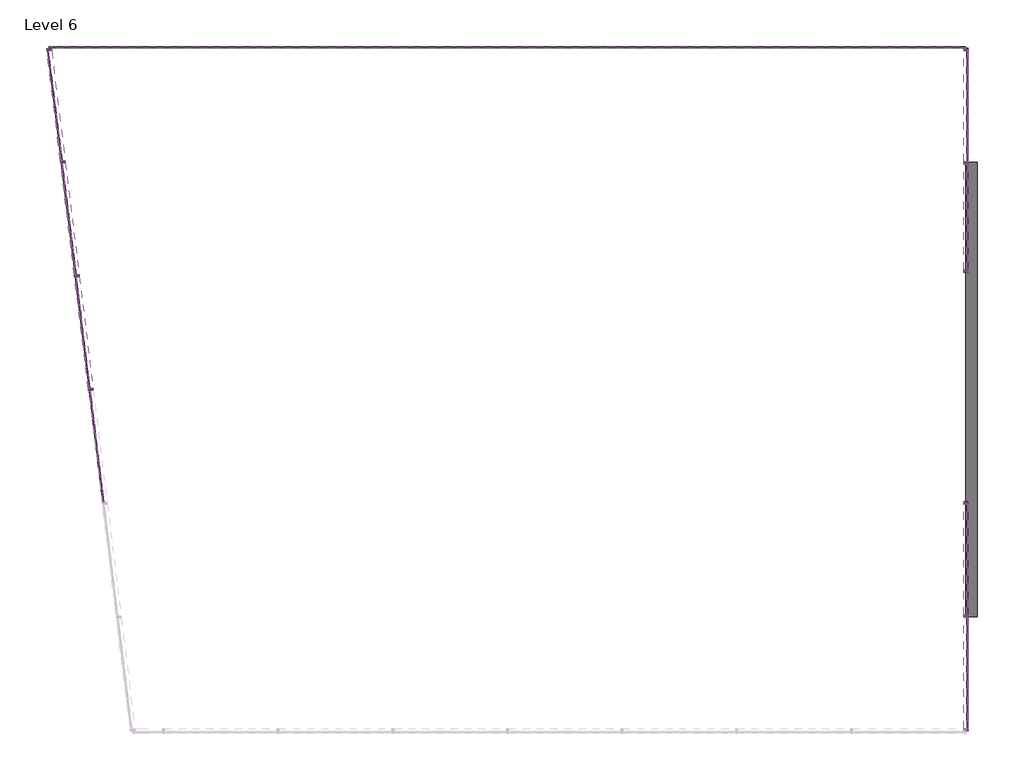
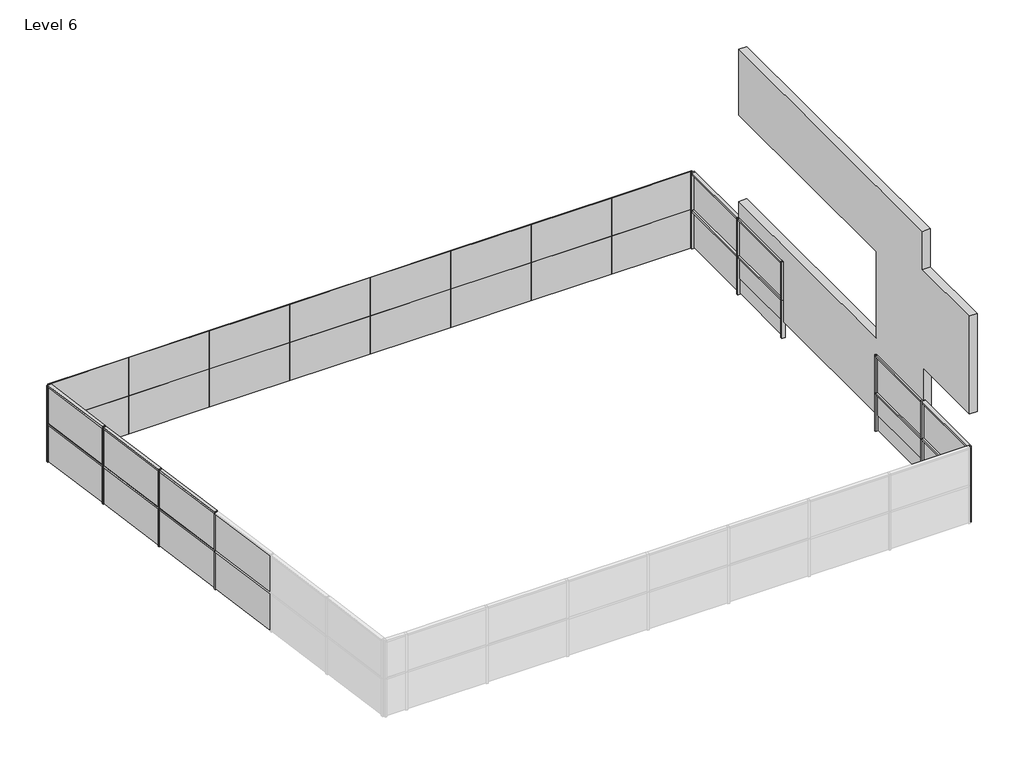
# One storey, part 2 of 2: 34 members, 32 plates, 1 proxy.
"""IFC4 building model written with IfcOpenShell, lengths in millimetres."""

from ifc_helpers import new_model, si_unit, origin, place, context, project, spatial, transform, mapped, element, save
from components import generic_models_3_generic_models_1_fe68d0d7, member_daa7a266, member_82905deb, member_19d0a4ec, member_8cef0660, member_4491d118, member_46bdb8c2, member_1b94d493, system_panel_glazed_1e57f9bb, system_panel_glazed_37f15d2e, system_panel_glazed_e46d4b42, system_panel_glazed_2a6c68b7, system_panel_glazed_7fb1fc2b, system_panel_glazed_d483336f

model = new_model("IFC4")

# Units and contexts
model_context = context("Model", 3, world=origin())
ifc_project = project(units=[si_unit("LENGTHUNIT", "METRE", prefix="MILLI")], contexts=[model_context])

# Site, building, storey
site = spatial("IfcSite", under=ifc_project)
building = spatial("IfcBuilding", under=site)
storey = spatial("IfcBuildingStorey", under=building, Name="Level 6", Elevation=15240.0)

# Proxy
placement = place(None, origin())
generic_models_3_generic_models_1_shape = generic_models_3_generic_models_1_fe68d0d7(model_context)
element("IfcBuildingElementProxy", 1, Name="Generic Models 3 : Generic Models 1", ObjectType="Generic Models 3 : Generic Models 1", at=placement, inside=storey, context=model_context, shape_type="MappedRepresentation", body=[
    mapped(generic_models_3_generic_models_1_shape, transform((0.0, 0.0, 17373.6), x_axis=(1.0, 0.0, 0.0), y_axis=(0.0, 1.0, 0.0), z_axis=(0.0, 0.0, 1.0))),
])

# Members
member_shape = member_daa7a266(model_context)
element("IfcMember", 2, ObjectType="Rectangular Mullion : 2.5\" x 5\" rectangular", at=placement, inside=storey, context=model_context, shape_type="MappedRepresentation", body=[
    mapped(member_shape, transform((13902.5156363, -946.6363705, 18288.0), x_axis=(0.0, 0.0, 1.0), y_axis=(1.0, 0.0, 0.0), z_axis=(0.0, 1.0, 0.0))),
])
element("IfcMember", 3, ObjectType="Rectangular Mullion : 2.5\" x 5\" rectangular", at=placement, inside=storey, context=model_context, shape_type="MappedRepresentation", body=[
    mapped(member_shape, transform((13902.5156363, -3962.8863708, 18288.0), x_axis=(0.0, 0.0, 1.0), y_axis=(1.0, 0.0, 0.0), z_axis=(0.0, 1.0, 0.0))),
])
element("IfcMember", 4, ObjectType="Rectangular Mullion : 2.5\" x 5\" rectangular", at=placement, inside=storey, context=model_context, shape_type="MappedRepresentation", body=[
    mapped(member_shape, transform((13902.5156363, 11109.0476508, 18288.0), x_axis=(0.0, 0.0, 1.0), y_axis=(1.0, 0.0, 0.0), z_axis=(0.0, 1.0, 0.0))),
])
member_2_shape = member_82905deb(model_context)
element("IfcMember", 5, ObjectType="Rectangular Mullion : 2.5\" x 5\" rectangular", at=placement, inside=storey, context=model_context, shape_type="MappedRepresentation", body=[
    mapped(member_2_shape, transform((13902.5156363, -3931.1363708, 18288.0), x_axis=(0.0, -1.0, 0.0), y_axis=(1.0, 0.0, 0.0), z_axis=(0.0, 0.0, 1.0))),
])
element("IfcMember", 6, ObjectType="Rectangular Mullion : 2.5\" x 5\" rectangular", at=placement, inside=storey, context=model_context, shape_type="MappedRepresentation", body=[
    mapped(member_2_shape, transform((13902.5156363, 8124.5476505, 18288.0), x_axis=(0.0, -1.0, 0.0), y_axis=(1.0, 0.0, 0.0), z_axis=(0.0, 0.0, 1.0))),
])
member_3_shape = member_19d0a4ec(model_context)
element("IfcMember", 7, ObjectType="Rectangular Mullion : 2.5\" x 5\" rectangular", at=placement, inside=storey, context=model_context, shape_type="MappedRepresentation", body=[
    mapped(member_3_shape, transform((-10113.8959567, 8178.7803212, 16764.0), x_axis=(0.0, 0.0, 1.0), y_axis=(-0.9925461516413222, -0.12186934340514609, 0.0), z_axis=(0.12186934340514609, -0.9925461516413222, 0.0))),
])
element("IfcMember", 8, ObjectType="Rectangular Mullion : 2.5\" x 5\" rectangular", at=placement, inside=storey, context=model_context, shape_type="MappedRepresentation", body=[
    mapped(member_3_shape, transform((-10113.8959567, 8178.7803212, 18288.0), x_axis=(0.0, 0.0, 1.0), y_axis=(-0.9925461516413222, -0.12186934340514617, 0.0), z_axis=(0.12186934340514617, -0.9925461516413222, 0.0))),
])
element("IfcMember", 9, ObjectType="Rectangular Mullion : 2.5\" x 5\" rectangular", at=placement, inside=storey, context=model_context, shape_type="MappedRepresentation", body=[
    mapped(member_3_shape, transform((13902.5156363, -946.6363705, 16764.0), x_axis=(0.0, 0.0, 1.0), y_axis=(1.0, 0.0, 0.0), z_axis=(0.0, 1.0, 0.0))),
])
element("IfcMember", 10, ObjectType="Rectangular Mullion : 2.5\" x 5\" rectangular", at=placement, inside=storey, context=model_context, shape_type="MappedRepresentation", body=[
    mapped(member_3_shape, transform((13902.5156363, -3962.8863708, 16764.0), x_axis=(0.0, 0.0, 1.0), y_axis=(1.0, 0.0, 0.0), z_axis=(0.0, 1.0, 0.0))),
])
element("IfcMember", 11, ObjectType="Rectangular Mullion : 2.5\" x 5\" rectangular", at=placement, inside=storey, context=model_context, shape_type="MappedRepresentation", body=[
    mapped(member_3_shape, transform((13902.5156363, 11109.0476508, 16764.0), x_axis=(0.0, 0.0, 1.0), y_axis=(1.0, 0.0, 0.0), z_axis=(0.0, 1.0, 0.0))),
])
member_4_shape = member_8cef0660(model_context)
element("IfcMember", 12, ObjectType="Rectangular Mullion : 2.5\" x 5\" rectangular", at=placement, inside=storey, context=model_context, shape_type="MappedRepresentation", body=[
    mapped(member_4_shape, transform((-9370.9804393, 2128.2189808, 16764.0), x_axis=(0.0, 0.0, 1.0), y_axis=(-0.9925461516413223, -0.12186934340514563, 0.0), z_axis=(0.12186934340514562, -0.9925461516413222, 0.0))),
])
element("IfcMember", 13, ObjectType="Rectangular Mullion : 2.5\" x 5\" rectangular", at=placement, inside=storey, context=model_context, shape_type="MappedRepresentation", body=[
    mapped(member_4_shape, transform((-9742.438198, 5153.499651, 16764.0), x_axis=(0.0, 0.0, 1.0), y_axis=(-0.9925461516413222, -0.12186934340514602, 0.0), z_axis=(0.12186934340514602, -0.9925461516413222, 0.0))),
])
element("IfcMember", 14, ObjectType="Rectangular Mullion : 2.5\" x 5\" rectangular", at=placement, inside=storey, context=model_context, shape_type="MappedRepresentation", body=[
    mapped(member_4_shape, transform((-9370.9804393, 2128.2189808, 18288.0), x_axis=(0.0, 0.0, 1.0), y_axis=(-0.9925461516413222, -0.12186934340514592, 0.0), z_axis=(0.12186934340514592, -0.9925461516413222, 0.0))),
])
element("IfcMember", 15, ObjectType="Rectangular Mullion : 2.5\" x 5\" rectangular", at=placement, inside=storey, context=model_context, shape_type="MappedRepresentation", body=[
    mapped(member_4_shape, transform((-9742.438198, 5153.499651, 18288.0), x_axis=(0.0, 0.0, 1.0), y_axis=(-0.9925461516413222, -0.1218693434051457, 0.0), z_axis=(0.1218693434051457, -0.9925461516413222, 0.0))),
])
element("IfcMember", 16, ObjectType="Rectangular Mullion : 2.5\" x 5\" rectangular", at=placement, inside=storey, context=model_context, shape_type="MappedRepresentation", body=[
    mapped(member_2_shape, transform((-9367.1110876, 2096.7056405, 16764.0), x_axis=(-0.1218693434051459, 0.9925461516413222, 0.0), y_axis=(-0.9925461516413222, -0.1218693434051459, 0.0), z_axis=(0.0, 0.0, 1.0))),
])
element("IfcMember", 17, ObjectType="Rectangular Mullion : 2.5\" x 5\" rectangular", at=placement, inside=storey, context=model_context, shape_type="MappedRepresentation", body=[
    mapped(member_2_shape, transform((-9367.1110876, 2096.7056405, 18288.0), x_axis=(-0.1218693434051459, 0.9925461516413222, 0.0), y_axis=(-0.9925461516413222, -0.1218693434051459, 0.0), z_axis=(0.0, 0.0, 1.0))),
])
element("IfcMember", 18, ObjectType="Rectangular Mullion : 2.5\" x 5\" rectangular", at=placement, inside=storey, context=model_context, shape_type="MappedRepresentation", body=[
    mapped(member_2_shape, transform((-9738.5688463, 5121.9863107, 16764.0), x_axis=(-0.1218693434051459, 0.9925461516413222, 0.0), y_axis=(-0.9925461516413222, -0.1218693434051459, 0.0), z_axis=(0.0, 0.0, 1.0))),
])
element("IfcMember", 19, ObjectType="Rectangular Mullion : 2.5\" x 5\" rectangular", at=placement, inside=storey, context=model_context, shape_type="MappedRepresentation", body=[
    mapped(member_2_shape, transform((-9738.5688463, 5121.9863107, 18288.0), x_axis=(-0.1218693434051459, 0.9925461516413222, 0.0), y_axis=(-0.9925461516413222, -0.1218693434051459, 0.0), z_axis=(0.0, 0.0, 1.0))),
])
element("IfcMember", 20, ObjectType="Rectangular Mullion : 2.5\" x 5\" rectangular", at=placement, inside=storey, context=model_context, shape_type="MappedRepresentation", body=[
    mapped(member_2_shape, transform((-10110.026605, 8147.2669809, 16764.0), x_axis=(-0.1218693434051459, 0.9925461516413222, 0.0), y_axis=(-0.9925461516413222, -0.1218693434051459, 0.0), z_axis=(0.0, 0.0, 1.0))),
])
element("IfcMember", 21, ObjectType="Rectangular Mullion : 2.5\" x 5\" rectangular", at=placement, inside=storey, context=model_context, shape_type="MappedRepresentation", body=[
    mapped(member_2_shape, transform((-10110.026605, 8147.2669809, 18288.0), x_axis=(-0.1218693434051459, 0.9925461516413222, 0.0), y_axis=(-0.9925461516413222, -0.1218693434051459, 0.0), z_axis=(0.0, 0.0, 1.0))),
])
element("IfcMember", 22, ObjectType="Rectangular Mullion : 2.5\" x 5\" rectangular", at=placement, inside=storey, context=model_context, shape_type="MappedRepresentation", body=[
    mapped(member_2_shape, transform((13902.5156363, -3931.1363708, 16764.0), x_axis=(0.0, -1.0, 0.0), y_axis=(1.0, 0.0, 0.0), z_axis=(0.0, 0.0, 1.0))),
])
element("IfcMember", 23, ObjectType="Rectangular Mullion : 2.5\" x 5\" rectangular", at=placement, inside=storey, context=model_context, shape_type="MappedRepresentation", body=[
    mapped(member_2_shape, transform((13902.5156363, 8124.5476505, 16764.0), x_axis=(0.0, -1.0, 0.0), y_axis=(1.0, 0.0, 0.0), z_axis=(0.0, 0.0, 1.0))),
])
member_5_shape = member_4491d118(model_context)
element("IfcMember", 24, ObjectType="Rectangular Mullion : 2.5\" x 5\" rectangular", at=placement, inside=storey, context=model_context, shape_type="MappedRepresentation", body=[
    mapped(member_5_shape, transform((13902.5156363, -6979.1363705, 18288.0), x_axis=(0.0, -1.0, 0.0), y_axis=(1.0, 0.0, 0.0), z_axis=(0.0, 0.0, 1.0))),
])
element("IfcMember", 25, ObjectType="Rectangular Mullion : 2.5\" x 5\" rectangular", at=placement, inside=storey, context=model_context, shape_type="MappedRepresentation", body=[
    mapped(member_5_shape, transform((13902.5156363, 5212.8636295, 18288.0), x_axis=(0.0, -1.0, 0.0), y_axis=(1.0, 0.0, 0.0), z_axis=(0.0, 0.0, 1.0))),
])
element("IfcMember", 26, ObjectType="Rectangular Mullion : 2.5\" x 5\" rectangular", at=placement, inside=storey, context=model_context, shape_type="MappedRepresentation", body=[
    mapped(member_5_shape, transform((13902.5156363, -883.1363705, 15240.0), x_axis=(0.0, 1.0, 0.0), y_axis=(1.0, 0.0, 0.0), z_axis=(0.0, 0.0, -1.0))),
])
element("IfcMember", 27, ObjectType="Rectangular Mullion : 2.5\" x 5\" rectangular", at=placement, inside=storey, context=model_context, shape_type="MappedRepresentation", body=[
    mapped(member_5_shape, transform((13902.5156363, 11172.5476508, 15240.0), x_axis=(0.0, 1.0, 0.0), y_axis=(1.0, 0.0, 0.0), z_axis=(0.0, 0.0, -1.0))),
])
element("IfcMember", 28, ObjectType="Rectangular Mullion : 2.5\" x 5\" rectangular", at=placement, inside=storey, context=model_context, shape_type="MappedRepresentation", body=[
    mapped(member_5_shape, transform((13902.5156363, -883.1363705, 16764.0), x_axis=(0.0, 1.0, 0.0), y_axis=(1.0, 0.0, 0.0), z_axis=(0.0, 0.0, -1.0))),
])
element("IfcMember", 29, ObjectType="Rectangular Mullion : 2.5\" x 5\" rectangular", at=placement, inside=storey, context=model_context, shape_type="MappedRepresentation", body=[
    mapped(member_5_shape, transform((13902.5156363, 11172.5476508, 16764.0), x_axis=(0.0, 1.0, 0.0), y_axis=(1.0, 0.0, 0.0), z_axis=(0.0, 0.0, -1.0))),
])
element("IfcMember", 30, ObjectType="Rectangular Mullion : 2.5\" x 5\" rectangular", at=placement, inside=storey, context=model_context, shape_type="MappedRepresentation", body=[
    mapped(member_5_shape, transform((-10481.4843637, 11172.5476508, 16764.0), x_axis=(-0.1218693434051459, 0.9925461516413222, 0.0), y_axis=(-0.9925461516413222, -0.1218693434051459, 0.0), z_axis=(0.0, 0.0, 1.0))),
])
element("IfcMember", 31, ObjectType="Rectangular Mullion : 2.5\" x 5\" rectangular", at=placement, inside=storey, context=model_context, shape_type="MappedRepresentation", body=[
    mapped(member_5_shape, transform((-10481.4843637, 11172.5476508, 18288.0), x_axis=(-0.1218693434051459, 0.9925461516413222, 0.0), y_axis=(-0.9925461516413222, -0.1218693434051459, 0.0), z_axis=(0.0, 0.0, 1.0))),
])
element("IfcMember", 32, ObjectType="Rectangular Mullion : 2.5\" x 5\" rectangular", at=placement, inside=storey, context=model_context, shape_type="MappedRepresentation", body=[
    mapped(member_5_shape, transform((13902.5156363, -6979.1363705, 16764.0), x_axis=(0.0, -1.0, 0.0), y_axis=(1.0, 0.0, 0.0), z_axis=(0.0, 0.0, 1.0))),
])
element("IfcMember", 33, ObjectType="Rectangular Mullion : 2.5\" x 5\" rectangular", at=placement, inside=storey, context=model_context, shape_type="MappedRepresentation", body=[
    mapped(member_5_shape, transform((13902.5156363, 5212.8636295, 16764.0), x_axis=(0.0, -1.0, 0.0), y_axis=(1.0, 0.0, 0.0), z_axis=(0.0, 0.0, 1.0))),
])
member_6_shape = member_46bdb8c2(model_context)
element("IfcMember", 34, ObjectType="Rectangular Mullion : 2.5\" x 5\" rectangular", at=placement, inside=storey, context=model_context, shape_type="MappedRepresentation", body=[
    mapped(member_6_shape, transform((13902.5156363, 8092.7976505, 16764.0), x_axis=(0.0, 0.0, 1.0), y_axis=(1.0, 0.0, 0.0), z_axis=(0.0, 1.0, 0.0))),
])
member_7_shape = member_1b94d493(model_context)
element("IfcMember", 35, ObjectType="Rectangular Mullion : 2.5\" x 5\" rectangular", at=placement, inside=storey, context=model_context, shape_type="MappedRepresentation", body=[
    mapped(member_7_shape, transform((13902.5156363, 8092.7976505, 18288.0), x_axis=(0.0, 0.0, 1.0), y_axis=(1.0, 0.0, 0.0), z_axis=(0.0, 1.0, 0.0))),
])

# Plates
system_panel_glazed_shape = system_panel_glazed_1e57f9bb(model_context)
element("IfcPlate", 36, ObjectType="System Panel : Glazed", at=placement, inside=storey, context=model_context, shape_type="MappedRepresentation", body=[
    mapped(system_panel_glazed_shape, transform((-8957.4843636, 11172.5476508, 15240.0), x_axis=(1.0, 0.0, 0.0), y_axis=(0.0, 1.0, 0.0), z_axis=(0.0, 0.0, 1.0))),
])
element("IfcPlate", 37, ObjectType="System Panel : Glazed", at=placement, inside=storey, context=model_context, shape_type="MappedRepresentation", body=[
    mapped(system_panel_glazed_shape, transform((-5909.4843634, 11172.5476508, 15240.0), x_axis=(1.0, 0.0, 0.0), y_axis=(0.0, 1.0, 0.0), z_axis=(0.0, 0.0, 1.0))),
])
element("IfcPlate", 38, ObjectType="System Panel : Glazed", at=placement, inside=storey, context=model_context, shape_type="MappedRepresentation", body=[
    mapped(system_panel_glazed_shape, transform((-2861.4843634, 11172.5476508, 15240.0), x_axis=(1.0, 0.0, 0.0), y_axis=(0.0, 1.0, 0.0), z_axis=(0.0, 0.0, 1.0))),
])
element("IfcPlate", 39, ObjectType="System Panel : Glazed", at=placement, inside=storey, context=model_context, shape_type="MappedRepresentation", body=[
    mapped(system_panel_glazed_shape, transform((186.5156366, 11172.5476508, 15240.0), x_axis=(1.0, 0.0, 0.0), y_axis=(0.0, 1.0, 0.0), z_axis=(0.0, 0.0, 1.0))),
])
element("IfcPlate", 40, ObjectType="System Panel : Glazed", at=placement, inside=storey, context=model_context, shape_type="MappedRepresentation", body=[
    mapped(system_panel_glazed_shape, transform((3234.5156366, 11172.5476508, 15240.0), x_axis=(1.0, 0.0, 0.0), y_axis=(0.0, 1.0, 0.0), z_axis=(0.0, 0.0, 1.0))),
])
element("IfcPlate", 41, ObjectType="System Panel : Glazed", at=placement, inside=storey, context=model_context, shape_type="MappedRepresentation", body=[
    mapped(system_panel_glazed_shape, transform((6282.5156366, 11172.5476508, 15240.0), x_axis=(1.0, 0.0, 0.0), y_axis=(0.0, 1.0, 0.0), z_axis=(0.0, 0.0, 1.0))),
])
element("IfcPlate", 42, ObjectType="System Panel : Glazed", at=placement, inside=storey, context=model_context, shape_type="MappedRepresentation", body=[
    mapped(system_panel_glazed_shape, transform((9330.5156366, 11172.5476508, 15240.0), x_axis=(1.0, 0.0, 0.0), y_axis=(0.0, 1.0, 0.0), z_axis=(0.0, 0.0, 1.0))),
])
element("IfcPlate", 43, ObjectType="System Panel : Glazed", at=placement, inside=storey, context=model_context, shape_type="MappedRepresentation", body=[
    mapped(system_panel_glazed_shape, transform((12378.5156364, 11172.5476508, 15240.0), x_axis=(1.0, 0.0, 0.0), y_axis=(0.0, 1.0, 0.0), z_axis=(0.0, 0.0, 1.0))),
])
element("IfcPlate", 44, ObjectType="System Panel : Glazed", at=placement, inside=storey, context=model_context, shape_type="MappedRepresentation", body=[
    mapped(system_panel_glazed_shape, transform((-8957.4843636, 11172.5476508, 16764.0), x_axis=(1.0, 0.0, 0.0), y_axis=(0.0, 1.0, 0.0), z_axis=(0.0, 0.0, 1.0))),
])
element("IfcPlate", 45, ObjectType="System Panel : Glazed", at=placement, inside=storey, context=model_context, shape_type="MappedRepresentation", body=[
    mapped(system_panel_glazed_shape, transform((-5909.4843634, 11172.5476508, 16764.0), x_axis=(1.0, 0.0, 0.0), y_axis=(0.0, 1.0, 0.0), z_axis=(0.0, 0.0, 1.0))),
])
element("IfcPlate", 46, ObjectType="System Panel : Glazed", at=placement, inside=storey, context=model_context, shape_type="MappedRepresentation", body=[
    mapped(system_panel_glazed_shape, transform((-2861.4843634, 11172.5476508, 16764.0), x_axis=(1.0, 0.0, 0.0), y_axis=(0.0, 1.0, 0.0), z_axis=(0.0, 0.0, 1.0))),
])
element("IfcPlate", 47, ObjectType="System Panel : Glazed", at=placement, inside=storey, context=model_context, shape_type="MappedRepresentation", body=[
    mapped(system_panel_glazed_shape, transform((186.5156366, 11172.5476508, 16764.0), x_axis=(1.0, 0.0, 0.0), y_axis=(0.0, 1.0, 0.0), z_axis=(0.0, 0.0, 1.0))),
])
element("IfcPlate", 48, ObjectType="System Panel : Glazed", at=placement, inside=storey, context=model_context, shape_type="MappedRepresentation", body=[
    mapped(system_panel_glazed_shape, transform((3234.5156366, 11172.5476508, 16764.0), x_axis=(1.0, 0.0, 0.0), y_axis=(0.0, 1.0, 0.0), z_axis=(0.0, 0.0, 1.0))),
])
element("IfcPlate", 49, ObjectType="System Panel : Glazed", at=placement, inside=storey, context=model_context, shape_type="MappedRepresentation", body=[
    mapped(system_panel_glazed_shape, transform((6282.5156366, 11172.5476508, 16764.0), x_axis=(1.0, 0.0, 0.0), y_axis=(0.0, 1.0, 0.0), z_axis=(0.0, 0.0, 1.0))),
])
element("IfcPlate", 50, ObjectType="System Panel : Glazed", at=placement, inside=storey, context=model_context, shape_type="MappedRepresentation", body=[
    mapped(system_panel_glazed_shape, transform((9330.5156366, 11172.5476508, 16764.0), x_axis=(1.0, 0.0, 0.0), y_axis=(0.0, 1.0, 0.0), z_axis=(0.0, 0.0, 1.0))),
])
element("IfcPlate", 51, ObjectType="System Panel : Glazed", at=placement, inside=storey, context=model_context, shape_type="MappedRepresentation", body=[
    mapped(system_panel_glazed_shape, transform((12378.5156364, 11172.5476508, 16764.0), x_axis=(1.0, 0.0, 0.0), y_axis=(0.0, 1.0, 0.0), z_axis=(0.0, 0.0, 1.0))),
])
system_panel_glazed_2_shape = system_panel_glazed_37f15d2e(model_context)
element("IfcPlate", 52, ObjectType="System Panel : Glazed", at=placement, inside=storey, context=model_context, shape_type="MappedRepresentation", body=[
    mapped(system_panel_glazed_2_shape, transform((13902.5156363, -2423.0113706, 16795.75), x_axis=(0.0, -1.0, 0.0), y_axis=(1.0, 0.0, 0.0), z_axis=(0.0, 0.0, 1.0))),
])
element("IfcPlate", 53, ObjectType="System Panel : Glazed", at=placement, inside=storey, context=model_context, shape_type="MappedRepresentation", body=[
    mapped(system_panel_glazed_2_shape, transform((13902.5156363, -5439.2613706, 16795.75), x_axis=(0.0, -1.0, 0.0), y_axis=(1.0, 0.0, 0.0), z_axis=(0.0, 0.0, 1.0))),
])
element("IfcPlate", 54, ObjectType="System Panel : Glazed", at=placement, inside=storey, context=model_context, shape_type="MappedRepresentation", body=[
    mapped(system_panel_glazed_2_shape, transform((13902.5156363, 9632.6726506, 16795.75), x_axis=(0.0, -1.0, 0.0), y_axis=(1.0, 0.0, 0.0), z_axis=(0.0, 0.0, 1.0))),
])
system_panel_glazed_3_shape = system_panel_glazed_e46d4b42(model_context)
element("IfcPlate", 55, ObjectType="System Panel : Glazed", at=placement, inside=storey, context=model_context, shape_type="MappedRepresentation", body=[
    mapped(system_panel_glazed_3_shape, transform((13902.5156363, -2423.0113706, 15271.75), x_axis=(0.0, -1.0, 0.0), y_axis=(1.0, 0.0, 0.0), z_axis=(0.0, 0.0, 1.0))),
])
element("IfcPlate", 56, ObjectType="System Panel : Glazed", at=placement, inside=storey, context=model_context, shape_type="MappedRepresentation", body=[
    mapped(system_panel_glazed_3_shape, transform((13902.5156363, -5439.2613706, 15271.75), x_axis=(0.0, -1.0, 0.0), y_axis=(1.0, 0.0, 0.0), z_axis=(0.0, 0.0, 1.0))),
])
element("IfcPlate", 57, ObjectType="System Panel : Glazed", at=placement, inside=storey, context=model_context, shape_type="MappedRepresentation", body=[
    mapped(system_panel_glazed_3_shape, transform((13902.5156363, 9632.6726506, 15271.75), x_axis=(0.0, -1.0, 0.0), y_axis=(1.0, 0.0, 0.0), z_axis=(0.0, 0.0, 1.0))),
])
element("IfcPlate", 58, ObjectType="System Panel : Glazed", at=placement, inside=storey, context=model_context, shape_type="MappedRepresentation", body=[
    mapped(system_panel_glazed_3_shape, transform((-10293.8208085, 9644.1506457, 15271.75), x_axis=(-0.1218693434051459, 0.9925461516413222, 0.0), y_axis=(-0.9925461516413222, -0.1218693434051459, 0.0), z_axis=(0.0, 0.0, 1.0))),
])
element("IfcPlate", 59, ObjectType="System Panel : Glazed", at=placement, inside=storey, context=model_context, shape_type="MappedRepresentation", body=[
    mapped(system_panel_glazed_3_shape, transform((-10293.8208085, 9644.1506457, 16795.75), x_axis=(-0.1218693434051459, 0.9925461516413222, 0.0), y_axis=(-0.9925461516413222, -0.1218693434051459, 0.0), z_axis=(0.0, 0.0, 1.0))),
])
system_panel_glazed_4_shape = system_panel_glazed_2a6c68b7(model_context)
element("IfcPlate", 60, ObjectType="System Panel : Glazed", at=placement, inside=storey, context=model_context, shape_type="MappedRepresentation", body=[
    mapped(system_panel_glazed_4_shape, transform((-9181.3822083, 584.0653054, 15271.75), x_axis=(-0.1218693434051459, 0.9925461516413222, 0.0), y_axis=(-0.9925461516413222, -0.1218693434051459, 0.0), z_axis=(0.0, 0.0, 1.0))),
])
element("IfcPlate", 61, ObjectType="System Panel : Glazed", at=placement, inside=storey, context=model_context, shape_type="MappedRepresentation", body=[
    mapped(system_panel_glazed_4_shape, transform((-9552.839967, 3609.3459756, 15271.75), x_axis=(-0.1218693434051459, 0.9925461516413222, 0.0), y_axis=(-0.9925461516413222, -0.1218693434051459, 0.0), z_axis=(0.0, 0.0, 1.0))),
])
element("IfcPlate", 62, ObjectType="System Panel : Glazed", at=placement, inside=storey, context=model_context, shape_type="MappedRepresentation", body=[
    mapped(system_panel_glazed_4_shape, transform((-9924.2977257, 6634.6266458, 15271.75), x_axis=(-0.1218693434051459, 0.9925461516413222, 0.0), y_axis=(-0.9925461516413222, -0.1218693434051459, 0.0), z_axis=(0.0, 0.0, 1.0))),
])
element("IfcPlate", 63, ObjectType="System Panel : Glazed", at=placement, inside=storey, context=model_context, shape_type="MappedRepresentation", body=[
    mapped(system_panel_glazed_4_shape, transform((-9181.3822083, 584.0653054, 16795.75), x_axis=(-0.1218693434051459, 0.9925461516413222, 0.0), y_axis=(-0.9925461516413222, -0.1218693434051459, 0.0), z_axis=(0.0, 0.0, 1.0))),
])
element("IfcPlate", 64, ObjectType="System Panel : Glazed", at=placement, inside=storey, context=model_context, shape_type="MappedRepresentation", body=[
    mapped(system_panel_glazed_4_shape, transform((-9552.839967, 3609.3459756, 16795.75), x_axis=(-0.1218693434051459, 0.9925461516413222, 0.0), y_axis=(-0.9925461516413222, -0.1218693434051459, 0.0), z_axis=(0.0, 0.0, 1.0))),
])
element("IfcPlate", 65, ObjectType="System Panel : Glazed", at=placement, inside=storey, context=model_context, shape_type="MappedRepresentation", body=[
    mapped(system_panel_glazed_4_shape, transform((-9924.2977257, 6634.6266458, 16795.75), x_axis=(-0.1218693434051459, 0.9925461516413222, 0.0), y_axis=(-0.9925461516413222, -0.1218693434051459, 0.0), z_axis=(0.0, 0.0, 1.0))),
])
system_panel_glazed_5_shape = system_panel_glazed_7fb1fc2b(model_context)
element("IfcPlate", 66, ObjectType="System Panel : Glazed", at=placement, inside=storey, context=model_context, shape_type="MappedRepresentation", body=[
    mapped(system_panel_glazed_5_shape, transform((13902.5156363, 6684.58064, 16795.75), x_axis=(0.0, -1.0, 0.0), y_axis=(1.0, 0.0, 0.0), z_axis=(0.0, 0.0, 1.0))),
])
system_panel_glazed_6_shape = system_panel_glazed_d483336f(model_context)
element("IfcPlate", 67, ObjectType="System Panel : Glazed", at=placement, inside=storey, context=model_context, shape_type="MappedRepresentation", body=[
    mapped(system_panel_glazed_6_shape, transform((13902.5156363, 6684.58064, 15271.75), x_axis=(0.0, -1.0, 0.0), y_axis=(1.0, 0.0, 0.0), z_axis=(0.0, 0.0, 1.0))),
])

save(model, "model.ifc")

# Revit data of these elements
# Type "Rectangular Mullion : 2.5\" x 5\" rectangular"
#   built-in parameter 1007304 = 0.416667 (stored number, unit not read)
#   built-in parameter 1007301 = 0.104167 (stored number, unit not read)
#   built-in parameter 1007300 = 0.104167 (stored number, unit not read)
# Type "System Panel : Glazed"
#   Construction Type Id = "GSP4R"
#   Analytic Construction = "1/8 in Pilkington single glazing"
#   Visual Light Transmittance = 0.9
#   Solar Heat Gain Coefficient = 0.86
#   Heat Transfer Coefficient (U) = 1.18115 BTU/(h·ft²·°F)
#   Define Thermal Properties by = 1
# Element 1 (IfcBuildingElementProxy, "Generic Models 3 : Generic Models 1")
#   Phase Created = New Construction
# Elements 2, 3, 4, 5, 6, 7, 8, 9, 10, 11, 12, 13, 14, 15, 16, 17, 18, 19, 20, 21, 22, 23, 24, 25, 26, 27, 28, 29, 30, 31, 32, 33, 34, 35 (IfcMember, "Rectangular Mullion : 2.5\" x 5\" rectangular")
#   Phase Created = New Construction
#   Materials on its faces: "Aluminum"
# Elements 36, 37, 38, 39, 40, 41, 42, 43, 44, 45, 46, 47, 48, 49, 50, 51, 52, 53, 54, 55, 56, 57, 58, 59, 60, 61, 62, 63, 64, 65, 66, 67 (IfcPlate, "System Panel : Glazed")
#   Phase Created = New Construction
#   Materials on its faces: "Glass"
# Materials
#   "Aluminum": class "Metal", colour RGB 247 247 247, transparency 0, Description = "Aluminum 6061", Cost = 0
#   "Glass": class "Glass", colour RGB 0 128 192, transparency 0.75, Description = "Soda Lime Glass", Cost = 0
